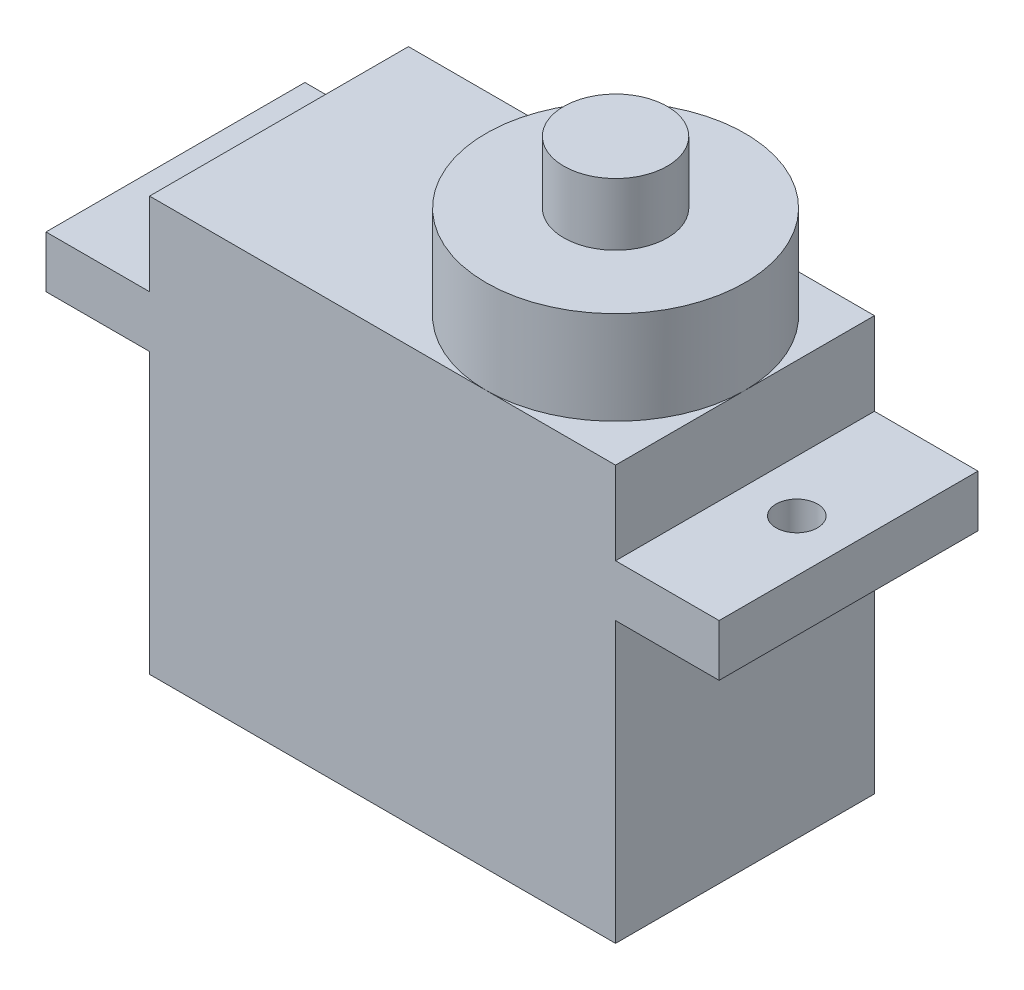
ISO-10303-21;
HEADER;
FILE_DESCRIPTION(('STEP AP214'),'2;1');
FILE_NAME('part.step','',(''),(''),'','','');
FILE_SCHEMA(('AUTOMOTIVE_DESIGN { 1 0 10303 214 1 1 1 1 }'));
ENDSEC;
DATA;
#1=APPLICATION_CONTEXT('core data for automotive mechanical design processes');
#2=APPLICATION_PROTOCOL_DEFINITION('international standard','automotive_design',2000,#1);
#3=PRODUCT_CONTEXT('',#1,'mechanical');
#4=PRODUCT('Part','Part','',(#3));
#5=PRODUCT_RELATED_PRODUCT_CATEGORY('part','',(#4));
#6=PRODUCT_DEFINITION_FORMATION('','',#4);
#7=PRODUCT_DEFINITION_CONTEXT('part definition',#1,'design');
#8=PRODUCT_DEFINITION('design','',#6,#7);
#9=PRODUCT_DEFINITION_SHAPE('','',#8);
#10=(LENGTH_UNIT() NAMED_UNIT(*) SI_UNIT(.MILLI.,.METRE.));
#11=(NAMED_UNIT(*) PLANE_ANGLE_UNIT() SI_UNIT($,.RADIAN.));
#12=(NAMED_UNIT(*) SI_UNIT($,.STERADIAN.) SOLID_ANGLE_UNIT());
#13=UNCERTAINTY_MEASURE_WITH_UNIT(LENGTH_MEASURE(1.E-05),#10,'distance_accuracy_value','');
#14=(GEOMETRIC_REPRESENTATION_CONTEXT(3) GLOBAL_UNCERTAINTY_ASSIGNED_CONTEXT((#13)) GLOBAL_UNIT_ASSIGNED_CONTEXT((#10,
#11,#12)) REPRESENTATION_CONTEXT('',''));
#15=CARTESIAN_POINT('',(0.,0.,0.));
#16=DIRECTION('',(0.,0.,1.));
#17=DIRECTION('',(1.,0.,0.));
#18=AXIS2_PLACEMENT_3D('',#15,#16,#17);
#19=CARTESIAN_POINT('',(22.5,0.,12.5));
#20=DIRECTION('',(0.,-1.,0.));
#21=DIRECTION('',(0.,0.,-1.));
#22=AXIS2_PLACEMENT_3D('',#19,#20,#21);
#23=PLANE('',#22);
#24=CARTESIAN_POINT('',(16.25,0.,6.25));
#25=DIRECTION('',(0.,1.,0.));
#26=DIRECTION('',(0.,0.,1.));
#27=AXIS2_PLACEMENT_3D('',#24,#25,#26);
#28=CIRCLE('',#27,6.25);
#29=CARTESIAN_POINT('',(16.25,0.,12.5));
#30=VERTEX_POINT('',#29);
#31=CARTESIAN_POINT('',(22.5,0.,6.25));
#32=VERTEX_POINT('',#31);
#33=EDGE_CURVE('E161',#30,#32,#28,.T.);
#34=ORIENTED_EDGE('',*,*,#33,.F.);
#35=DIRECTION('',(-1.,0.,0.));
#36=VECTOR('',#35,1.);
#37=CARTESIAN_POINT('',(22.5,0.,12.5));
#38=LINE('',#37,#36);
#39=CARTESIAN_POINT('',(22.5,0.,12.5));
#40=VERTEX_POINT('',#39);
#41=EDGE_CURVE('E144',#40,#30,#38,.T.);
#42=ORIENTED_EDGE('',*,*,#41,.F.);
#43=DIRECTION('',(0.,0.,-1.));
#44=VECTOR('',#43,1.);
#45=CARTESIAN_POINT('',(22.5,0.,12.5));
#46=LINE('',#45,#44);
#47=EDGE_CURVE('E165',#40,#32,#46,.T.);
#48=ORIENTED_EDGE('',*,*,#47,.T.);
#49=EDGE_LOOP('',(#34,#42,#48));
#50=FACE_BOUND('',#49,.T.);
#51=ADVANCED_FACE('F44',(#50),#23,.F.);
#52=CARTESIAN_POINT('',(16.25,0.,0.));
#53=VERTEX_POINT('',#52);
#54=EDGE_CURVE('E53',#32,#53,#28,.T.);
#55=ORIENTED_EDGE('',*,*,#54,.F.);
#56=CARTESIAN_POINT('',(22.5,0.,0.));
#57=VERTEX_POINT('',#56);
#58=EDGE_CURVE('E204',#32,#57,#46,.T.);
#59=ORIENTED_EDGE('',*,*,#58,.T.);
#60=DIRECTION('',(-1.,0.,0.));
#61=VECTOR('',#60,1.);
#62=CARTESIAN_POINT('',(22.5,0.,0.));
#63=LINE('',#62,#61);
#64=EDGE_CURVE('E202',#57,#53,#63,.T.);
#65=ORIENTED_EDGE('',*,*,#64,.T.);
#66=EDGE_LOOP('',(#55,#59,#65));
#67=FACE_BOUND('',#66,.T.);
#68=ADVANCED_FACE('F288',(#67),#23,.F.);
#69=EDGE_CURVE('E68',#53,#30,#28,.T.);
#70=ORIENTED_EDGE('',*,*,#69,.F.);
#71=CARTESIAN_POINT('',(0.,0.,0.));
#72=VERTEX_POINT('',#71);
#73=EDGE_CURVE('E173',#53,#72,#63,.T.);
#74=ORIENTED_EDGE('',*,*,#73,.T.);
#75=DIRECTION('',(0.,0.,-1.));
#76=VECTOR('',#75,1.);
#77=CARTESIAN_POINT('',(0.,0.,12.5));
#78=LINE('',#77,#76);
#79=CARTESIAN_POINT('',(0.,0.,12.5));
#80=VERTEX_POINT('',#79);
#81=EDGE_CURVE('E47',#80,#72,#78,.T.);
#82=ORIENTED_EDGE('',*,*,#81,.F.);
#83=EDGE_CURVE('E150',#30,#80,#38,.T.);
#84=ORIENTED_EDGE('',*,*,#83,.F.);
#85=EDGE_LOOP('',(#70,#74,#82,#84));
#86=FACE_BOUND('',#85,.T.);
#87=ADVANCED_FACE('F50',(#86),#23,.F.);
#88=CARTESIAN_POINT('',(0.,0.,12.5));
#89=DIRECTION('',(1.,0.,0.));
#90=DIRECTION('',(0.,0.,-1.));
#91=AXIS2_PLACEMENT_3D('',#88,#89,#90);
#92=PLANE('',#91);
#93=DIRECTION('',(0.,-1.,0.));
#94=VECTOR('',#93,1.);
#95=CARTESIAN_POINT('',(0.,0.,0.));
#96=LINE('',#95,#94);
#97=CARTESIAN_POINT('',(0.,-4.,0.));
#98=VERTEX_POINT('',#97);
#99=EDGE_CURVE('E210',#72,#98,#96,.T.);
#100=ORIENTED_EDGE('',*,*,#99,.T.);
#101=DIRECTION('',(0.,0.,-1.));
#102=VECTOR('',#101,1.);
#103=CARTESIAN_POINT('',(0.,-4.,12.5));
#104=LINE('',#103,#102);
#105=CARTESIAN_POINT('',(0.,-4.,12.5));
#106=VERTEX_POINT('',#105);
#107=EDGE_CURVE('E169',#106,#98,#104,.T.);
#108=ORIENTED_EDGE('',*,*,#107,.F.);
#109=DIRECTION('',(0.,-1.,0.));
#110=VECTOR('',#109,1.);
#111=CARTESIAN_POINT('',(0.,0.,12.5));
#112=LINE('',#111,#110);
#113=EDGE_CURVE('E154',#80,#106,#112,.T.);
#114=ORIENTED_EDGE('',*,*,#113,.F.);
#115=ORIENTED_EDGE('',*,*,#81,.T.);
#116=EDGE_LOOP('',(#100,#108,#114,#115));
#117=FACE_BOUND('',#116,.T.);
#118=ADVANCED_FACE('F281',(#117),#92,.F.);
#119=CARTESIAN_POINT('',(0.,-4.,12.5));
#120=DIRECTION('',(0.,-1.,0.));
#121=DIRECTION('',(0.,0.,-1.));
#122=AXIS2_PLACEMENT_3D('',#119,#120,#121);
#123=PLANE('',#122);
#124=CARTESIAN_POINT('',(-2.5,-4.,6.25));
#125=DIRECTION('',(0.,1.,0.));
#126=DIRECTION('',(0.,0.,1.));
#127=AXIS2_PLACEMENT_3D('',#124,#125,#126);
#128=CIRCLE('',#127,1.);
#129=CARTESIAN_POINT('',(-2.5,-4.,7.25));
#130=VERTEX_POINT('',#129);
#131=EDGE_CURVE('E182',#130,#130,#128,.T.);
#132=ORIENTED_EDGE('',*,*,#131,.F.);
#133=EDGE_LOOP('',(#132));
#134=FACE_BOUND('',#133,.T.);
#135=DIRECTION('',(-1.,0.,0.));
#136=VECTOR('',#135,1.);
#137=CARTESIAN_POINT('',(0.,-4.,0.));
#138=LINE('',#137,#136);
#139=CARTESIAN_POINT('',(-5.,-4.,0.));
#140=VERTEX_POINT('',#139);
#141=EDGE_CURVE('E207',#98,#140,#138,.T.);
#142=ORIENTED_EDGE('',*,*,#141,.T.);
#143=DIRECTION('',(0.,0.,-1.));
#144=VECTOR('',#143,1.);
#145=CARTESIAN_POINT('',(-5.,-4.,12.5));
#146=LINE('',#145,#144);
#147=CARTESIAN_POINT('',(-5.,-4.,12.5));
#148=VERTEX_POINT('',#147);
#149=EDGE_CURVE('E255',#148,#140,#146,.T.);
#150=ORIENTED_EDGE('',*,*,#149,.F.);
#151=DIRECTION('',(-1.,0.,0.));
#152=VECTOR('',#151,1.);
#153=CARTESIAN_POINT('',(0.,-4.,12.5));
#154=LINE('',#153,#152);
#155=EDGE_CURVE('E183',#106,#148,#154,.T.);
#156=ORIENTED_EDGE('',*,*,#155,.F.);
#157=ORIENTED_EDGE('',*,*,#107,.T.);
#158=EDGE_LOOP('',(#142,#150,#156,#157));
#159=FACE_BOUND('',#158,.T.);
#160=ADVANCED_FACE('F261',(#134,#159),#123,.F.);
#161=CARTESIAN_POINT('',(-5.,-4.,12.5));
#162=DIRECTION('',(1.,0.,0.));
#163=DIRECTION('',(0.,0.,-1.));
#164=AXIS2_PLACEMENT_3D('',#161,#162,#163);
#165=PLANE('',#164);
#166=DIRECTION('',(0.,-1.,0.));
#167=VECTOR('',#166,1.);
#168=CARTESIAN_POINT('',(-5.,-4.,0.));
#169=LINE('',#168,#167);
#170=CARTESIAN_POINT('',(-5.,-6.5,0.));
#171=VERTEX_POINT('',#170);
#172=EDGE_CURVE('E211',#140,#171,#169,.T.);
#173=ORIENTED_EDGE('',*,*,#172,.T.);
#174=DIRECTION('',(0.,0.,-1.));
#175=VECTOR('',#174,1.);
#176=CARTESIAN_POINT('',(-5.,-6.5,12.5));
#177=LINE('',#176,#175);
#178=CARTESIAN_POINT('',(-5.,-6.5,12.5));
#179=VERTEX_POINT('',#178);
#180=EDGE_CURVE('E253',#179,#171,#177,.T.);
#181=ORIENTED_EDGE('',*,*,#180,.F.);
#182=DIRECTION('',(0.,-1.,0.));
#183=VECTOR('',#182,1.);
#184=CARTESIAN_POINT('',(-5.,-4.,12.5));
#185=LINE('',#184,#183);
#186=EDGE_CURVE('E187',#148,#179,#185,.T.);
#187=ORIENTED_EDGE('',*,*,#186,.F.);
#188=ORIENTED_EDGE('',*,*,#149,.T.);
#189=EDGE_LOOP('',(#173,#181,#187,#188));
#190=FACE_BOUND('',#189,.T.);
#191=ADVANCED_FACE('F272',(#190),#165,.F.);
#192=CARTESIAN_POINT('',(-5.,-6.5,12.5));
#193=DIRECTION('',(0.,1.,0.));
#194=DIRECTION('',(0.,0.,1.));
#195=AXIS2_PLACEMENT_3D('',#192,#193,#194);
#196=PLANE('',#195);
#197=CARTESIAN_POINT('',(-2.5,-6.5,6.25));
#198=DIRECTION('',(0.,1.,0.));
#199=DIRECTION('',(0.,0.,1.));
#200=AXIS2_PLACEMENT_3D('',#197,#198,#199);
#201=CIRCLE('',#200,1.);
#202=CARTESIAN_POINT('',(-2.5,-6.5,7.25));
#203=VERTEX_POINT('',#202);
#204=EDGE_CURVE('E179',#203,#203,#201,.T.);
#205=ORIENTED_EDGE('',*,*,#204,.T.);
#206=EDGE_LOOP('',(#205));
#207=FACE_BOUND('',#206,.T.);
#208=DIRECTION('',(1.,0.,0.));
#209=VECTOR('',#208,1.);
#210=CARTESIAN_POINT('',(-5.,-6.5,0.));
#211=LINE('',#210,#209);
#212=CARTESIAN_POINT('',(0.,-6.5,0.));
#213=VERTEX_POINT('',#212);
#214=EDGE_CURVE('E213',#171,#213,#211,.T.);
#215=ORIENTED_EDGE('',*,*,#214,.T.);
#216=DIRECTION('',(0.,0.,-1.));
#217=VECTOR('',#216,1.);
#218=CARTESIAN_POINT('',(0.,-6.5,12.5));
#219=LINE('',#218,#217);
#220=CARTESIAN_POINT('',(0.,-6.5,12.5));
#221=VERTEX_POINT('',#220);
#222=EDGE_CURVE('E249',#221,#213,#219,.T.);
#223=ORIENTED_EDGE('',*,*,#222,.F.);
#224=DIRECTION('',(1.,0.,0.));
#225=VECTOR('',#224,1.);
#226=CARTESIAN_POINT('',(-5.,-6.5,12.5));
#227=LINE('',#226,#225);
#228=EDGE_CURVE('E188',#179,#221,#227,.T.);
#229=ORIENTED_EDGE('',*,*,#228,.F.);
#230=ORIENTED_EDGE('',*,*,#180,.T.);
#231=EDGE_LOOP('',(#215,#223,#229,#230));
#232=FACE_BOUND('',#231,.T.);
#233=ADVANCED_FACE('F280',(#207,#232),#196,.F.);
#234=CARTESIAN_POINT('',(0.,-6.5,12.5));
#235=DIRECTION('',(1.,0.,0.));
#236=DIRECTION('',(0.,0.,-1.));
#237=AXIS2_PLACEMENT_3D('',#234,#235,#236);
#238=PLANE('',#237);
#239=DIRECTION('',(0.,-1.,0.));
#240=VECTOR('',#239,1.);
#241=CARTESIAN_POINT('',(0.,-6.5,0.));
#242=LINE('',#241,#240);
#243=CARTESIAN_POINT('',(0.,-20.,0.));
#244=VERTEX_POINT('',#243);
#245=EDGE_CURVE('E214',#213,#244,#242,.T.);
#246=ORIENTED_EDGE('',*,*,#245,.T.);
#247=DIRECTION('',(0.,0.,-1.));
#248=VECTOR('',#247,1.);
#249=CARTESIAN_POINT('',(0.,-20.,12.5));
#250=LINE('',#249,#248);
#251=CARTESIAN_POINT('',(0.,-20.,12.5));
#252=VERTEX_POINT('',#251);
#253=EDGE_CURVE('E245',#252,#244,#250,.T.);
#254=ORIENTED_EDGE('',*,*,#253,.F.);
#255=DIRECTION('',(0.,-1.,0.));
#256=VECTOR('',#255,1.);
#257=CARTESIAN_POINT('',(0.,-6.5,12.5));
#258=LINE('',#257,#256);
#259=EDGE_CURVE('E191',#221,#252,#258,.T.);
#260=ORIENTED_EDGE('',*,*,#259,.F.);
#261=ORIENTED_EDGE('',*,*,#222,.T.);
#262=EDGE_LOOP('',(#246,#254,#260,#261));
#263=FACE_BOUND('',#262,.T.);
#264=ADVANCED_FACE('F328',(#263),#238,.F.);
#265=CARTESIAN_POINT('',(0.,-20.,12.5));
#266=DIRECTION('',(0.,1.,0.));
#267=DIRECTION('',(0.,0.,1.));
#268=AXIS2_PLACEMENT_3D('',#265,#266,#267);
#269=PLANE('',#268);
#270=DIRECTION('',(1.,0.,0.));
#271=VECTOR('',#270,1.);
#272=CARTESIAN_POINT('',(0.,-20.,0.));
#273=LINE('',#272,#271);
#274=CARTESIAN_POINT('',(22.5,-20.,0.));
#275=VERTEX_POINT('',#274);
#276=EDGE_CURVE('E220',#244,#275,#273,.T.);
#277=ORIENTED_EDGE('',*,*,#276,.T.);
#278=DIRECTION('',(0.,0.,-1.));
#279=VECTOR('',#278,1.);
#280=CARTESIAN_POINT('',(22.5,-20.,12.5));
#281=LINE('',#280,#279);
#282=CARTESIAN_POINT('',(22.5,-20.,12.5));
#283=VERTEX_POINT('',#282);
#284=EDGE_CURVE('E242',#283,#275,#281,.T.);
#285=ORIENTED_EDGE('',*,*,#284,.F.);
#286=DIRECTION('',(1.,0.,0.));
#287=VECTOR('',#286,1.);
#288=CARTESIAN_POINT('',(0.,-20.,12.5));
#289=LINE('',#288,#287);
#290=EDGE_CURVE('E194',#252,#283,#289,.T.);
#291=ORIENTED_EDGE('',*,*,#290,.F.);
#292=ORIENTED_EDGE('',*,*,#253,.T.);
#293=EDGE_LOOP('',(#277,#285,#291,#292));
#294=FACE_BOUND('',#293,.T.);
#295=ADVANCED_FACE('F338',(#294),#269,.F.);
#296=CARTESIAN_POINT('',(22.5,-20.,12.5));
#297=DIRECTION('',(-1.,0.,0.));
#298=DIRECTION('',(0.,0.,1.));
#299=AXIS2_PLACEMENT_3D('',#296,#297,#298);
#300=PLANE('',#299);
#301=DIRECTION('',(0.,1.,0.));
#302=VECTOR('',#301,1.);
#303=CARTESIAN_POINT('',(22.5,-20.,0.));
#304=LINE('',#303,#302);
#305=CARTESIAN_POINT('',(22.5,-6.5,0.));
#306=VERTEX_POINT('',#305);
#307=EDGE_CURVE('E218',#275,#306,#304,.T.);
#308=ORIENTED_EDGE('',*,*,#307,.T.);
#309=DIRECTION('',(0.,0.,-1.));
#310=VECTOR('',#309,1.);
#311=CARTESIAN_POINT('',(22.5,-6.5,12.5));
#312=LINE('',#311,#310);
#313=CARTESIAN_POINT('',(22.5,-6.5,12.5));
#314=VERTEX_POINT('',#313);
#315=EDGE_CURVE('E239',#314,#306,#312,.T.);
#316=ORIENTED_EDGE('',*,*,#315,.F.);
#317=DIRECTION('',(0.,1.,0.));
#318=VECTOR('',#317,1.);
#319=CARTESIAN_POINT('',(22.5,-20.,12.5));
#320=LINE('',#319,#318);
#321=EDGE_CURVE('E195',#283,#314,#320,.T.);
#322=ORIENTED_EDGE('',*,*,#321,.F.);
#323=ORIENTED_EDGE('',*,*,#284,.T.);
#324=EDGE_LOOP('',(#308,#316,#322,#323));
#325=FACE_BOUND('',#324,.T.);
#326=ADVANCED_FACE('F348',(#325),#300,.F.);
#327=CARTESIAN_POINT('',(22.5,-6.5,12.5));
#328=DIRECTION('',(0.,1.,0.));
#329=DIRECTION('',(0.,0.,1.));
#330=AXIS2_PLACEMENT_3D('',#327,#328,#329);
#331=PLANE('',#330);
#332=CARTESIAN_POINT('',(25.,-6.5,6.25));
#333=DIRECTION('',(0.,1.,0.));
#334=DIRECTION('',(0.,0.,1.));
#335=AXIS2_PLACEMENT_3D('',#332,#333,#334);
#336=CIRCLE('',#335,1.);
#337=CARTESIAN_POINT('',(25.,-6.5,7.25));
#338=VERTEX_POINT('',#337);
#339=EDGE_CURVE('E171',#338,#338,#336,.T.);
#340=ORIENTED_EDGE('',*,*,#339,.T.);
#341=EDGE_LOOP('',(#340));
#342=FACE_BOUND('',#341,.T.);
#343=DIRECTION('',(1.,0.,0.));
#344=VECTOR('',#343,1.);
#345=CARTESIAN_POINT('',(22.5,-6.5,0.));
#346=LINE('',#345,#344);
#347=CARTESIAN_POINT('',(27.5,-6.5,0.));
#348=VERTEX_POINT('',#347);
#349=EDGE_CURVE('E222',#306,#348,#346,.T.);
#350=ORIENTED_EDGE('',*,*,#349,.T.);
#351=DIRECTION('',(0.,0.,-1.));
#352=VECTOR('',#351,1.);
#353=CARTESIAN_POINT('',(27.5,-6.5,12.5));
#354=LINE('',#353,#352);
#355=CARTESIAN_POINT('',(27.5,-6.5,12.5));
#356=VERTEX_POINT('',#355);
#357=EDGE_CURVE('E237',#356,#348,#354,.T.);
#358=ORIENTED_EDGE('',*,*,#357,.F.);
#359=DIRECTION('',(1.,0.,0.));
#360=VECTOR('',#359,1.);
#361=CARTESIAN_POINT('',(22.5,-6.5,12.5));
#362=LINE('',#361,#360);
#363=EDGE_CURVE('E197',#314,#356,#362,.T.);
#364=ORIENTED_EDGE('',*,*,#363,.F.);
#365=ORIENTED_EDGE('',*,*,#315,.T.);
#366=EDGE_LOOP('',(#350,#358,#364,#365));
#367=FACE_BOUND('',#366,.T.);
#368=ADVANCED_FACE('F363',(#342,#367),#331,.F.);
#369=CARTESIAN_POINT('',(27.5,-6.5,12.5));
#370=DIRECTION('',(-1.,0.,0.));
#371=DIRECTION('',(0.,0.,1.));
#372=AXIS2_PLACEMENT_3D('',#369,#370,#371);
#373=PLANE('',#372);
#374=DIRECTION('',(0.,1.,0.));
#375=VECTOR('',#374,1.);
#376=CARTESIAN_POINT('',(27.5,-6.5,0.));
#377=LINE('',#376,#375);
#378=CARTESIAN_POINT('',(27.5,-4.,0.));
#379=VERTEX_POINT('',#378);
#380=EDGE_CURVE('E224',#348,#379,#377,.T.);
#381=ORIENTED_EDGE('',*,*,#380,.T.);
#382=DIRECTION('',(0.,0.,-1.));
#383=VECTOR('',#382,1.);
#384=CARTESIAN_POINT('',(27.5,-4.,12.5));
#385=LINE('',#384,#383);
#386=CARTESIAN_POINT('',(27.5,-4.,12.5));
#387=VERTEX_POINT('',#386);
#388=EDGE_CURVE('E234',#387,#379,#385,.T.);
#389=ORIENTED_EDGE('',*,*,#388,.F.);
#390=DIRECTION('',(0.,1.,0.));
#391=VECTOR('',#390,1.);
#392=CARTESIAN_POINT('',(27.5,-6.5,12.5));
#393=LINE('',#392,#391);
#394=EDGE_CURVE('E200',#356,#387,#393,.T.);
#395=ORIENTED_EDGE('',*,*,#394,.F.);
#396=ORIENTED_EDGE('',*,*,#357,.T.);
#397=EDGE_LOOP('',(#381,#389,#395,#396));
#398=FACE_BOUND('',#397,.T.);
#399=ADVANCED_FACE('F375',(#398),#373,.F.);
#400=CARTESIAN_POINT('',(27.5,-4.,12.5));
#401=DIRECTION('',(0.,-1.,0.));
#402=DIRECTION('',(0.,0.,-1.));
#403=AXIS2_PLACEMENT_3D('',#400,#401,#402);
#404=PLANE('',#403);
#405=CARTESIAN_POINT('',(25.,-4.,6.25));
#406=DIRECTION('',(0.,1.,0.));
#407=DIRECTION('',(0.,0.,1.));
#408=AXIS2_PLACEMENT_3D('',#405,#406,#407);
#409=CIRCLE('',#408,1.);
#410=CARTESIAN_POINT('',(25.,-4.,7.25));
#411=VERTEX_POINT('',#410);
#412=EDGE_CURVE('E175',#411,#411,#409,.T.);
#413=ORIENTED_EDGE('',*,*,#412,.F.);
#414=EDGE_LOOP('',(#413));
#415=FACE_BOUND('',#414,.T.);
#416=DIRECTION('',(-1.,0.,0.));
#417=VECTOR('',#416,1.);
#418=CARTESIAN_POINT('',(27.5,-4.,0.));
#419=LINE('',#418,#417);
#420=CARTESIAN_POINT('',(22.5,-4.,0.));
#421=VERTEX_POINT('',#420);
#422=EDGE_CURVE('E223',#379,#421,#419,.T.);
#423=ORIENTED_EDGE('',*,*,#422,.T.);
#424=DIRECTION('',(0.,0.,-1.));
#425=VECTOR('',#424,1.);
#426=CARTESIAN_POINT('',(22.5,-4.,12.5));
#427=LINE('',#426,#425);
#428=CARTESIAN_POINT('',(22.5,-4.,12.5));
#429=VERTEX_POINT('',#428);
#430=EDGE_CURVE('E230',#429,#421,#427,.T.);
#431=ORIENTED_EDGE('',*,*,#430,.F.);
#432=DIRECTION('',(-1.,0.,0.));
#433=VECTOR('',#432,1.);
#434=CARTESIAN_POINT('',(27.5,-4.,12.5));
#435=LINE('',#434,#433);
#436=EDGE_CURVE('E203',#387,#429,#435,.T.);
#437=ORIENTED_EDGE('',*,*,#436,.F.);
#438=ORIENTED_EDGE('',*,*,#388,.T.);
#439=EDGE_LOOP('',(#423,#431,#437,#438));
#440=FACE_BOUND('',#439,.T.);
#441=ADVANCED_FACE('F385',(#415,#440),#404,.F.);
#442=CARTESIAN_POINT('',(22.5,-4.,12.5));
#443=DIRECTION('',(-1.,0.,0.));
#444=DIRECTION('',(0.,0.,1.));
#445=AXIS2_PLACEMENT_3D('',#442,#443,#444);
#446=PLANE('',#445);
#447=DIRECTION('',(0.,1.,0.));
#448=VECTOR('',#447,1.);
#449=CARTESIAN_POINT('',(22.5,-4.,0.));
#450=LINE('',#449,#448);
#451=EDGE_CURVE('E157',#421,#57,#450,.T.);
#452=ORIENTED_EDGE('',*,*,#451,.T.);
#453=ORIENTED_EDGE('',*,*,#58,.F.);
#454=ORIENTED_EDGE('',*,*,#47,.F.);
#455=DIRECTION('',(0.,1.,0.));
#456=VECTOR('',#455,1.);
#457=CARTESIAN_POINT('',(22.5,-4.,12.5));
#458=LINE('',#457,#456);
#459=EDGE_CURVE('E147',#429,#40,#458,.T.);
#460=ORIENTED_EDGE('',*,*,#459,.F.);
#461=ORIENTED_EDGE('',*,*,#430,.T.);
#462=EDGE_LOOP('',(#452,#453,#454,#460,#461));
#463=FACE_BOUND('',#462,.T.);
#464=ADVANCED_FACE('F391',(#463),#446,.F.);
#465=CARTESIAN_POINT('',(0.,0.,12.5));
#466=DIRECTION('',(0.,0.,1.));
#467=DIRECTION('',(1.,0.,0.));
#468=AXIS2_PLACEMENT_3D('',#465,#466,#467);
#469=PLANE('',#468);
#470=ORIENTED_EDGE('',*,*,#41,.T.);
#471=ORIENTED_EDGE('',*,*,#83,.T.);
#472=ORIENTED_EDGE('',*,*,#113,.T.);
#473=ORIENTED_EDGE('',*,*,#155,.T.);
#474=ORIENTED_EDGE('',*,*,#186,.T.);
#475=ORIENTED_EDGE('',*,*,#228,.T.);
#476=ORIENTED_EDGE('',*,*,#259,.T.);
#477=ORIENTED_EDGE('',*,*,#290,.T.);
#478=ORIENTED_EDGE('',*,*,#321,.T.);
#479=ORIENTED_EDGE('',*,*,#363,.T.);
#480=ORIENTED_EDGE('',*,*,#394,.T.);
#481=ORIENTED_EDGE('',*,*,#436,.T.);
#482=ORIENTED_EDGE('',*,*,#459,.T.);
#483=EDGE_LOOP('',(#470,#471,#472,#473,#474,#475,#476,#477,#478,#479,#480,#481,#482));
#484=FACE_BOUND('',#483,.T.);
#485=ADVANCED_FACE('F148',(#484),#469,.T.);
#486=CARTESIAN_POINT('',(0.,0.,0.));
#487=DIRECTION('',(0.,0.,1.));
#488=DIRECTION('',(1.,0.,0.));
#489=AXIS2_PLACEMENT_3D('',#486,#487,#488);
#490=PLANE('',#489);
#491=ORIENTED_EDGE('',*,*,#64,.F.);
#492=ORIENTED_EDGE('',*,*,#451,.F.);
#493=ORIENTED_EDGE('',*,*,#422,.F.);
#494=ORIENTED_EDGE('',*,*,#380,.F.);
#495=ORIENTED_EDGE('',*,*,#349,.F.);
#496=ORIENTED_EDGE('',*,*,#307,.F.);
#497=ORIENTED_EDGE('',*,*,#276,.F.);
#498=ORIENTED_EDGE('',*,*,#245,.F.);
#499=ORIENTED_EDGE('',*,*,#214,.F.);
#500=ORIENTED_EDGE('',*,*,#172,.F.);
#501=ORIENTED_EDGE('',*,*,#141,.F.);
#502=ORIENTED_EDGE('',*,*,#99,.F.);
#503=ORIENTED_EDGE('',*,*,#73,.F.);
#504=EDGE_LOOP('',(#491,#492,#493,#494,#495,#496,#497,#498,#499,#500,#501,#502,#503));
#505=FACE_BOUND('',#504,.T.);
#506=ADVANCED_FACE('F268',(#505),#490,.F.);
#507=CARTESIAN_POINT('',(25.,-6.5,6.25));
#508=DIRECTION('',(0.,1.,0.));
#509=DIRECTION('',(0.,0.,1.));
#510=AXIS2_PLACEMENT_3D('',#507,#508,#509);
#511=CYLINDRICAL_SURFACE('',#510,1.);
#512=ORIENTED_EDGE('',*,*,#339,.F.);
#513=EDGE_LOOP('',(#512));
#514=FACE_BOUND('',#513,.T.);
#515=ORIENTED_EDGE('',*,*,#412,.T.);
#516=EDGE_LOOP('',(#515));
#517=FACE_BOUND('',#516,.T.);
#518=ADVANCED_FACE('F417',(#514,#517),#511,.F.);
#519=CARTESIAN_POINT('',(-2.5,-6.5,6.25));
#520=DIRECTION('',(0.,1.,0.));
#521=DIRECTION('',(0.,0.,1.));
#522=AXIS2_PLACEMENT_3D('',#519,#520,#521);
#523=CYLINDRICAL_SURFACE('',#522,1.);
#524=ORIENTED_EDGE('',*,*,#204,.F.);
#525=EDGE_LOOP('',(#524));
#526=FACE_BOUND('',#525,.T.);
#527=ORIENTED_EDGE('',*,*,#131,.T.);
#528=EDGE_LOOP('',(#527));
#529=FACE_BOUND('',#528,.T.);
#530=ADVANCED_FACE('F422',(#526,#529),#523,.F.);
#531=CARTESIAN_POINT('',(16.25,4.5,6.25));
#532=DIRECTION('',(0.,-1.,0.));
#533=DIRECTION('',(0.,0.,-1.));
#534=AXIS2_PLACEMENT_3D('',#531,#532,#533);
#535=CYLINDRICAL_SURFACE('',#534,6.25);
#536=CARTESIAN_POINT('',(16.25,4.5,6.25));
#537=DIRECTION('',(0.,1.,0.));
#538=DIRECTION('',(0.,0.,1.));
#539=AXIS2_PLACEMENT_3D('',#536,#537,#538);
#540=CIRCLE('',#539,6.25);
#541=CARTESIAN_POINT('',(16.25,4.5,12.5));
#542=VERTEX_POINT('',#541);
#543=EDGE_CURVE('E163',#542,#542,#540,.T.);
#544=ORIENTED_EDGE('',*,*,#543,.F.);
#545=EDGE_LOOP('',(#544));
#546=FACE_BOUND('',#545,.T.);
#547=ORIENTED_EDGE('',*,*,#33,.T.);
#548=ORIENTED_EDGE('',*,*,#54,.T.);
#549=ORIENTED_EDGE('',*,*,#69,.T.);
#550=EDGE_LOOP('',(#547,#548,#549));
#551=FACE_BOUND('',#550,.T.);
#552=ADVANCED_FACE('F170',(#546,#551),#535,.T.);
#553=CARTESIAN_POINT('',(16.25,4.5,6.25));
#554=DIRECTION('',(0.,1.,0.));
#555=DIRECTION('',(0.,0.,1.));
#556=AXIS2_PLACEMENT_3D('',#553,#554,#555);
#557=PLANE('',#556);
#558=CARTESIAN_POINT('',(16.25,4.5,6.25));
#559=DIRECTION('',(0.,1.,0.));
#560=DIRECTION('',(0.,0.,1.));
#561=AXIS2_PLACEMENT_3D('',#558,#559,#560);
#562=CIRCLE('',#561,2.5);
#563=CARTESIAN_POINT('',(16.25,4.5,8.75));
#564=VERTEX_POINT('',#563);
#565=EDGE_CURVE('E11',#564,#564,#562,.T.);
#566=ORIENTED_EDGE('',*,*,#565,.F.);
#567=EDGE_LOOP('',(#566));
#568=FACE_BOUND('',#567,.T.);
#569=ORIENTED_EDGE('',*,*,#543,.T.);
#570=EDGE_LOOP('',(#569));
#571=FACE_BOUND('',#570,.T.);
#572=ADVANCED_FACE('F444',(#568,#571),#557,.T.);
#573=CARTESIAN_POINT('',(16.25,7.5,6.25));
#574=DIRECTION('',(0.,-1.,0.));
#575=DIRECTION('',(0.,0.,-1.));
#576=AXIS2_PLACEMENT_3D('',#573,#574,#575);
#577=CYLINDRICAL_SURFACE('',#576,2.5);
#578=CARTESIAN_POINT('',(16.25,7.5,6.25));
#579=DIRECTION('',(0.,1.,0.));
#580=DIRECTION('',(0.,0.,1.));
#581=AXIS2_PLACEMENT_3D('',#578,#579,#580);
#582=CIRCLE('',#581,2.5);
#583=CARTESIAN_POINT('',(16.25,7.5,8.75));
#584=VERTEX_POINT('',#583);
#585=EDGE_CURVE('E164',#584,#584,#582,.T.);
#586=ORIENTED_EDGE('',*,*,#585,.F.);
#587=EDGE_LOOP('',(#586));
#588=FACE_BOUND('',#587,.T.);
#589=ORIENTED_EDGE('',*,*,#565,.T.);
#590=EDGE_LOOP('',(#589));
#591=FACE_BOUND('',#590,.T.);
#592=ADVANCED_FACE('F454',(#588,#591),#577,.T.);
#593=CARTESIAN_POINT('',(16.25,7.5,6.25));
#594=DIRECTION('',(0.,1.,0.));
#595=DIRECTION('',(0.,0.,1.));
#596=AXIS2_PLACEMENT_3D('',#593,#594,#595);
#597=PLANE('',#596);
#598=ORIENTED_EDGE('',*,*,#585,.T.);
#599=EDGE_LOOP('',(#598));
#600=FACE_BOUND('',#599,.T.);
#601=ADVANCED_FACE('F464',(#600),#597,.T.);
#602=CLOSED_SHELL('',(#51,#68,#87,#118,#160,#191,#233,#264,#295,#326,#368,#399,#441,#464,#485,
#506,#518,#530,#552,#572,#592,#601));
#603=MANIFOLD_SOLID_BREP('B2',#602);
#604=ADVANCED_BREP_SHAPE_REPRESENTATION('',(#18,#603),#14);
#605=SHAPE_DEFINITION_REPRESENTATION(#9,#604);
ENDSEC;
END-ISO-10303-21;
